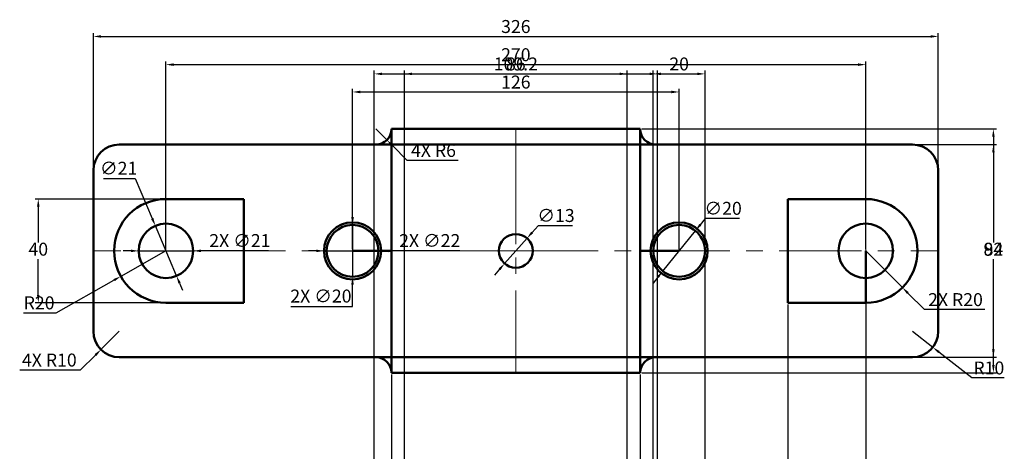
# Model space of a CAD drawing. Units: millimetres. Extents: x -44 to 350, y 28 to 429.
# Tile 2 of 2: x -44 to 336, y 262 to 429. Entities that reach past the tile are written whole.
import ezdxf

# ---------------------------------------------------------------- set-up
doc = ezdxf.new("R2010")
doc.units = ezdxf.units.MM
doc.linetypes.add('CENTER', pattern=[50.8, 31.75, -6.35, 6.35, -6.35])
for name, color, linetype, lineweight in [('M-CNTR', 1, 'CENTER', 18), ('M-DIMS', 2, 'Continuous', 25), ('M-OUTL', 7, 'Continuous', 50)]:
    doc.layers.add(name, color=color, linetype=linetype, lineweight=lineweight)
doc.styles.get("Standard").update_dxf_attribs({"font": 'arial.ttf'})
doc.dimstyles.new('ISO-25', dxfattribs={"dimtxt": 5, "dimasz": 3, "dimexe": 1.25, "dimexo": 0.625, "dimtad": 1, "dimtih": 1, "dimtoh": 1, "dimtxsty": 'Standard', "dimcen": 2.5, "dimadec": 0, "dimazin": 0, "dimtfac": 1, "dimtmove": 0, "dimatfit": 3, "dimfxl": 1, "dimarcsym": 0})

# ---------------------------------------------------------------- blocks, each defined once
blk = doc.blocks.new('*D20')
at = {"layer": 'Defpoints', "color": 0, "transparency": 16777216}
for p in [(310.7, 422.26), (-15.3, 370.57), (310.7, 370.57)]:
    blk.add_point(p, dxfattribs=at)
at = {"layer": 'M-DIMS', "color": 0, "lineweight": -2, "transparency": 16777216}
for p, q in [((-15.3, 371.19), (-15.3, 423.51)), ((-12.3, 422.26), (307.7, 422.26)), ((310.7, 371.19), (310.7, 423.51))]:
    blk.add_line(p, q, dxfattribs=at)
at = {"layer": 'M-DIMS', "color": 0, "transparency": 16777216}
for points in [[(-12.3, 422.76), (-12.3, 421.76), (-15.3, 422.26)], [(307.7, 422.76), (307.7, 421.76), (310.7, 422.26)]]:
    blk.add_solid(points, dxfattribs=at)
at = {"layer": 'M-DIMS', "color": 0, "transparency": 16777216, "insert": (147.7, 425.44), "char_height": 5, "attachment_point": 5}
blk.add_mtext('326', dxfattribs=at)
blk = doc.blocks.new('*D21')
at = {"layer": 'Defpoints', "color": 0, "transparency": 16777216}
for p in [(282.7, 411.39), (12.7, 339.57), (282.7, 339.57)]:
    blk.add_point(p, dxfattribs=at)
at = {"layer": 'M-DIMS', "color": 0, "lineweight": -2, "transparency": 16777216}
for p, q in [((12.7, 340.19), (12.7, 412.64)), ((15.7, 411.39), (279.7, 411.39)), ((282.7, 340.19), (282.7, 412.64))]:
    blk.add_line(p, q, dxfattribs=at)
at = {"layer": 'M-DIMS', "color": 0, "transparency": 16777216}
for points in [[(15.7, 411.89), (15.7, 410.89), (12.7, 411.39)], [(279.7, 411.89), (279.7, 410.89), (282.7, 411.39)]]:
    blk.add_solid(points, dxfattribs=at)
at = {"layer": 'M-DIMS', "color": 0, "transparency": 16777216, "insert": (147.7, 414.57), "char_height": 5, "attachment_point": 5}
blk.add_mtext('270', dxfattribs=at)
blk = doc.blocks.new('*D22')
at = {"layer": 'Defpoints', "color": 0, "transparency": 16777216}
for p in [(210.7, 400.84), (84.7, 339.57), (210.7, 339.57)]:
    blk.add_point(p, dxfattribs=at)
at = {"layer": 'M-DIMS', "color": 0, "lineweight": -2, "transparency": 16777216}
for p, q in [((84.7, 340.19), (84.7, 402.09)), ((87.7, 400.84), (207.7, 400.84)), ((210.7, 340.19), (210.7, 402.09))]:
    blk.add_line(p, q, dxfattribs=at)
at = {"layer": 'M-DIMS', "color": 0, "transparency": 16777216}
for points in [[(87.7, 401.34), (87.7, 400.34), (84.7, 400.84)], [(207.7, 401.34), (207.7, 400.34), (210.7, 400.84)]]:
    blk.add_solid(points, dxfattribs=at)
at = {"layer": 'M-DIMS', "color": 0, "transparency": 16777216, "insert": (147.7, 404.02), "char_height": 5, "attachment_point": 5}
blk.add_mtext('126', dxfattribs=at)
blk = doc.blocks.new('*D23')
at = {"layer": 'Defpoints', "color": 0, "transparency": 16777216}
for p in [(152.01, 344.43), (143.39, 334.7)]:
    blk.add_point(p, dxfattribs=at)
at = {"layer": 'M-DIMS', "color": 0, "lineweight": -2, "transparency": 16777216}
for p, q in [((156.27, 349.24), (154, 346.68)), ((169.5, 349.24), (156.27, 349.24)), ((143.39, 334.7), (152.01, 344.43)), ((141.4, 332.46), (139.41, 330.21))]:
    blk.add_line(p, q, dxfattribs=at)
at = {"layer": 'M-DIMS', "color": 0, "transparency": 16777216}
for points in [[(153.63, 347.01), (154.37, 346.35), (152.01, 344.43)], [(141.03, 332.79), (141.78, 332.13), (143.39, 334.7)]]:
    blk.add_solid(points, dxfattribs=at)
at = {"layer": 'M-DIMS', "color": 0, "transparency": 16777216, "insert": (163.2, 352.56), "char_height": 5, "attachment_point": 5}
blk.add_mtext('∅13', dxfattribs=at)
blk = doc.blocks.new('*D24')
at = {"layer": 'Defpoints', "color": 0, "transparency": 16777216}
for p in [(216.99, 347.34), (204.41, 331.79)]:
    blk.add_point(p, dxfattribs=at)
at = {"layer": 'M-DIMS', "color": 0, "lineweight": -2, "transparency": 16777216}
for p, q in [((220.77, 352.01), (218.88, 349.67)), ((233.98, 352.01), (220.77, 352.01)), ((204.41, 331.79), (216.99, 347.34)), ((202.52, 329.46), (200.64, 327.13))]:
    blk.add_line(p, q, dxfattribs=at)
at = {"layer": 'M-DIMS', "color": 0, "transparency": 16777216}
for points in [[(218.49, 349.99), (219.27, 349.36), (216.99, 347.34)], [(202.13, 329.78), (202.91, 329.15), (204.41, 331.79)]]:
    blk.add_solid(points, dxfattribs=at)
at = {"layer": 'M-DIMS', "color": 0, "transparency": 16777216, "insert": (227.68, 355.32), "char_height": 5, "attachment_point": 5}
blk.add_mtext('∅20', dxfattribs=at)
blk = doc.blocks.new('*D25')
at = {"layer": 'Defpoints', "color": 0, "transparency": 16777216}
for p in [(300.7, 308.57), (308.57, 302.39)]:
    blk.add_point(p, dxfattribs=at)
at = {"layer": 'M-DIMS', "color": 0, "lineweight": -2, "transparency": 16777216}
for p, q in [((300.7, 308.57), (308.57, 302.39)), ((323.61, 290.58), (310.93, 300.54)), ((336.16, 290.58), (323.61, 290.58))]:
    blk.add_line(p, q, dxfattribs=at)
at = {"layer": 'M-DIMS', "color": 0, "transparency": 16777216}
blk.add_solid([(311.23, 300.93), (310.62, 300.15), (308.57, 302.39)], dxfattribs=at)
at = {"layer": 'M-DIMS', "color": 0, "transparency": 16777216, "insert": (330.2, 293.76), "char_height": 5, "attachment_point": 5}
blk.add_mtext('R10', dxfattribs=at)
blk = doc.blocks.new('*D26')
at = {"layer": 'Defpoints', "color": 0, "transparency": 16777216}
for p in [(8.61, 349.24), (16.79, 329.9)]:
    blk.add_point(p, dxfattribs=at)
at = {"layer": 'M-DIMS', "color": 0, "lineweight": -2, "transparency": 16777216}
for p, q in [((-11.37, 367.47), (0.89, 367.47)), ((0.89, 367.47), (7.44, 352)), ((16.79, 329.9), (8.61, 349.24)), ((17.96, 327.14), (19.13, 324.37))]:
    blk.add_line(p, q, dxfattribs=at)
at = {"layer": 'M-DIMS', "color": 0, "transparency": 16777216}
for points in [[(7.9, 352.2), (6.98, 351.81), (8.61, 349.24)], [(18.42, 327.33), (17.5, 326.94), (16.79, 329.9)]]:
    blk.add_solid(points, dxfattribs=at)
at = {"layer": 'M-DIMS', "color": 0, "transparency": 16777216, "insert": (-5.55, 370.79), "char_height": 5, "attachment_point": 5}
blk.add_mtext('∅21', dxfattribs=at)
blk = doc.blocks.new('*D27')
at = {"layer": 'Defpoints', "color": 0, "transparency": 16777216}
for p in [(12.7, 339.57), (-4.72, 329.75)]:
    blk.add_point(p, dxfattribs=at)
at = {"layer": 'M-DIMS', "color": 0, "lineweight": -2, "transparency": 16777216}
for p, q in [((12.7, 339.57), (-4.72, 329.75)), ((-29.64, 315.7), (-7.34, 328.27)), ((-42.2, 315.7), (-29.64, 315.7))]:
    blk.add_line(p, q, dxfattribs=at)
at = {"layer": 'M-DIMS', "color": 0, "transparency": 16777216}
blk.add_solid([(-7.58, 328.71), (-7.09, 327.84), (-4.72, 329.75)], dxfattribs=at)
at = {"layer": 'M-DIMS', "color": 0, "transparency": 16777216, "insert": (-36.23, 318.88), "char_height": 5, "attachment_point": 5}
blk.add_mtext('R20', dxfattribs=at)
blk = doc.blocks.new('*D28')
at = {"layer": 'Defpoints', "color": 0, "transparency": 16777216}
for p in [(300.7, 380.57), (331.95, 380.57), (300.7, 298.57)]:
    blk.add_point(p, dxfattribs=at)
at = {"layer": 'M-DIMS', "color": 0, "lineweight": -2, "transparency": 16777216}
for p, q in [((301.33, 380.57), (333.2, 380.57)), ((331.95, 377.57), (331.95, 342.75)), ((331.95, 301.57), (331.95, 336.39)), ((301.33, 298.57), (333.2, 298.57))]:
    blk.add_line(p, q, dxfattribs=at)
at = {"layer": 'M-DIMS', "color": 0, "transparency": 16777216}
for points in [[(331.45, 377.57), (332.45, 377.57), (331.95, 380.57)], [(331.45, 301.57), (332.45, 301.57), (331.95, 298.57)]]:
    blk.add_solid(points, dxfattribs=at)
at = {"layer": 'M-DIMS', "color": 0, "transparency": 16777216, "insert": (331.95, 339.57), "char_height": 5, "attachment_point": 5}
blk.add_mtext('82', dxfattribs=at)
blk = doc.blocks.new('*D29')
at = {"layer": 'Defpoints', "color": 0, "transparency": 16777216}
for p in [(195.7, 386.57), (331.95, 386.57), (195.7, 292.57)]:
    blk.add_point(p, dxfattribs=at)
at = {"layer": 'M-DIMS', "color": 0, "lineweight": -2, "transparency": 16777216}
for p, q in [((196.33, 386.57), (333.2, 386.57)), ((331.95, 383.57), (331.95, 342.75)), ((331.95, 295.57), (331.95, 336.39)), ((196.33, 292.57), (333.2, 292.57))]:
    blk.add_line(p, q, dxfattribs=at)
at = {"layer": 'M-DIMS', "color": 0, "transparency": 16777216}
for points in [[(331.45, 383.57), (332.45, 383.57), (331.95, 386.57)], [(331.45, 295.57), (332.45, 295.57), (331.95, 292.57)]]:
    blk.add_solid(points, dxfattribs=at)
at = {"layer": 'M-DIMS', "color": 0, "transparency": 16777216, "insert": (331.95, 339.57), "char_height": 5, "attachment_point": 5}
blk.add_mtext('94', dxfattribs=at)
blk = doc.blocks.new('*D30')
at = {"layer": 'Defpoints', "color": 0, "transparency": 16777216}
for p in [(99.7, 292.57), (195.7, 292.57), (195.7, 28.91)]:
    blk.add_point(p, dxfattribs=at)
at = {"layer": 'M-DIMS', "color": 0, "lineweight": -2, "transparency": 16777216}
for p, q in [((99.7, 291.94), (99.7, 27.66)), ((195.7, 291.94), (195.7, 27.66)), ((102.7, 28.91), (192.7, 28.91))]:
    blk.add_line(p, q, dxfattribs=at)
at = {"layer": 'M-DIMS', "color": 0, "transparency": 16777216}
for points in [[(102.7, 29.41), (102.7, 28.41), (99.7, 28.91)], [(192.7, 29.41), (192.7, 28.41), (195.7, 28.91)]]:
    blk.add_solid(points, dxfattribs=at)
at = {"layer": 'M-DIMS', "color": 0, "transparency": 16777216, "insert": (147.7, 32.09), "char_height": 5, "attachment_point": 5}
blk.add_mtext('96', dxfattribs=at)
blk = doc.blocks.new('*D31')
at = {"layer": 'Defpoints', "color": 0, "transparency": 16777216}
for p in [(282.7, 339.57), (252.7, 319.57), (252.7, 28.91)]:
    blk.add_point(p, dxfattribs=at)
at = {"layer": 'M-DIMS', "color": 0, "lineweight": -2, "transparency": 16777216}
for p, q in [((282.7, 338.94), (282.7, 27.66)), ((252.7, 318.94), (252.7, 27.66)), ((279.7, 28.91), (255.7, 28.91))]:
    blk.add_line(p, q, dxfattribs=at)
at = {"layer": 'M-DIMS', "color": 0, "transparency": 16777216}
for points in [[(255.7, 29.41), (255.7, 28.41), (252.7, 28.91)], [(279.7, 29.41), (279.7, 28.41), (282.7, 28.91)]]:
    blk.add_solid(points, dxfattribs=at)
at = {"layer": 'M-DIMS', "color": 0, "transparency": 16777216, "insert": (267.7, 32.09), "char_height": 5, "attachment_point": 5}
blk.add_mtext('30', dxfattribs=at)
blk = doc.blocks.new('*D32')
at = {"layer": 'Defpoints', "color": 0, "transparency": 16777216}
for p in [(-36.55, 359.57), (42.7, 359.57), (42.7, 319.57)]:
    blk.add_point(p, dxfattribs=at)
at = {"layer": 'M-DIMS', "color": 0, "lineweight": -2, "transparency": 16777216}
for p, q in [((42.08, 359.57), (-37.8, 359.57)), ((-36.55, 356.57), (-36.55, 342.75)), ((-36.55, 322.57), (-36.55, 336.39)), ((42.08, 319.57), (-37.8, 319.57))]:
    blk.add_line(p, q, dxfattribs=at)
at = {"layer": 'M-DIMS', "color": 0, "transparency": 16777216}
for points in [[(-37.05, 356.57), (-36.05, 356.57), (-36.55, 359.57)], [(-37.05, 322.57), (-36.05, 322.57), (-36.55, 319.57)]]:
    blk.add_solid(points, dxfattribs=at)
at = {"layer": 'M-DIMS', "color": 0, "transparency": 16777216, "insert": (-36.55, 339.57), "char_height": 5, "attachment_point": 5}
blk.add_mtext('40', dxfattribs=at)
blk = doc.blocks.new('*D36')
at = {"layer": 'Defpoints', "color": 0, "transparency": 16777216}
for p in [(202.3, 407.82), (93.1, 177.16), (202.3, 177.16)]:
    blk.add_point(p, dxfattribs=at)
at = {"layer": 'M-DIMS', "color": 0, "lineweight": -2, "transparency": 16777216}
for p, q in [((93.1, 177.78), (93.1, 409.07)), ((96.1, 407.82), (199.3, 407.82)), ((202.3, 177.78), (202.3, 409.07))]:
    blk.add_line(p, q, dxfattribs=at)
at = {"layer": 'M-DIMS', "color": 0, "transparency": 16777216}
for points in [[(96.1, 408.32), (96.1, 407.32), (93.1, 407.82)], [(199.3, 408.32), (199.3, 407.32), (202.3, 407.82)]]:
    blk.add_solid(points, dxfattribs=at)
at = {"layer": 'M-DIMS', "color": 0, "transparency": 16777216, "insert": (147.7, 411), "char_height": 5, "attachment_point": 5}
blk.add_mtext('109.2', dxfattribs=at)
blk = doc.blocks.new('*D37')
at = {"layer": 'Defpoints', "color": 0, "transparency": 16777216}
for p in [(190.7, 407.82), (104.7, 131.22), (190.7, 131.22)]:
    blk.add_point(p, dxfattribs=at)
at = {"layer": 'M-DIMS', "color": 0, "lineweight": -2, "transparency": 16777216}
for p, q in [((104.7, 131.85), (104.7, 409.07)), ((107.7, 407.82), (187.7, 407.82)), ((190.7, 131.85), (190.7, 409.07))]:
    blk.add_line(p, q, dxfattribs=at)
at = {"layer": 'M-DIMS', "color": 0, "transparency": 16777216}
for points in [[(107.7, 408.32), (107.7, 407.32), (104.7, 407.82)], [(187.7, 408.32), (187.7, 407.32), (190.7, 407.82)]]:
    blk.add_solid(points, dxfattribs=at)
at = {"layer": 'M-DIMS', "color": 0, "transparency": 16777216, "insert": (147.7, 411), "char_height": 5, "attachment_point": 5}
blk.add_mtext('86', dxfattribs=at)
blk = doc.blocks.new('*D42')
at = {"layer": 'Defpoints', "color": 0, "transparency": 16777216}
for p in [(220.7, 407.82), (200.7, 78.16), (220.7, 78.16)]:
    blk.add_point(p, dxfattribs=at)
at = {"layer": 'M-DIMS', "color": 0, "lineweight": -2, "transparency": 16777216}
for p, q in [((200.7, 78.78), (200.7, 409.07)), ((203.7, 407.82), (217.7, 407.82)), ((220.7, 78.78), (220.7, 409.07))]:
    blk.add_line(p, q, dxfattribs=at)
at = {"layer": 'M-DIMS', "color": 0, "transparency": 16777216}
for points in [[(203.7, 408.32), (203.7, 407.32), (200.7, 407.82)], [(217.7, 408.32), (217.7, 407.32), (220.7, 407.82)]]:
    blk.add_solid(points, dxfattribs=at)
at = {"layer": 'M-DIMS', "color": 0, "transparency": 16777216, "insert": (210.7, 411), "char_height": 5, "attachment_point": 5}
blk.add_mtext('20', dxfattribs=at)
blk = doc.blocks.new('*D43')
at = {"layer": 'Defpoints', "color": 0, "transparency": 16777216}
for p in [(2.2, 339.57), (23.2, 339.57)]:
    blk.add_point(p, dxfattribs=at)
at = {"layer": 'M-DIMS', "color": 0, "lineweight": -2, "transparency": 16777216}
for p, q in [((-0.8, 339.57), (-3.8, 339.57)), ((2.2, 339.57), (23.2, 339.57)), ((29.5, 339.57), (26.2, 339.57)), ((52.33, 339.57), (29.5, 339.57))]:
    blk.add_line(p, q, dxfattribs=at)
at = {"layer": 'M-DIMS', "color": 0, "transparency": 16777216}
for points in [[(-0.8, 340.07), (-0.8, 339.07), (2.2, 339.57)], [(26.2, 340.07), (26.2, 339.07), (23.2, 339.57)]]:
    blk.add_solid(points, dxfattribs=at)
at = {"layer": 'M-DIMS', "color": 0, "transparency": 16777216, "insert": (41.23, 342.89), "char_height": 5, "attachment_point": 5}
blk.add_mtext('2X ∅21', dxfattribs=at)
blk = doc.blocks.new('*D44')
at = {"layer": 'Defpoints', "color": 0, "transparency": 16777216}
for p in [(73.7, 339.57), (95.7, 339.57)]:
    blk.add_point(p, dxfattribs=at)
at = {"layer": 'M-DIMS', "color": 0, "lineweight": -2, "transparency": 16777216}
for p, q in [((70.7, 339.57), (67.7, 339.57)), ((73.7, 339.57), (95.7, 339.57)), ((102.3, 339.57), (98.7, 339.57)), ((126.04, 339.57), (102.3, 339.57))]:
    blk.add_line(p, q, dxfattribs=at)
at = {"layer": 'M-DIMS', "color": 0, "transparency": 16777216}
for points in [[(70.7, 340.07), (70.7, 339.07), (73.7, 339.57)], [(98.7, 340.07), (98.7, 339.07), (95.7, 339.57)]]:
    blk.add_solid(points, dxfattribs=at)
at = {"layer": 'M-DIMS', "color": 0, "transparency": 16777216, "insert": (114.48, 342.89), "char_height": 5, "attachment_point": 5}
blk.add_mtext('2X ∅22', dxfattribs=at)
blk = doc.blocks.new('*D45')
at = {"layer": 'Defpoints', "color": 0, "transparency": 16777216}
for p in [(84.7, 349.57), (84.7, 329.57)]:
    blk.add_point(p, dxfattribs=at)
at = {"layer": 'M-DIMS', "color": 0, "lineweight": -2, "transparency": 16777216}
for p, q in [((84.7, 352.57), (84.7, 355.57)), ((84.7, 349.57), (84.7, 329.57)), ((84.7, 318.18), (84.7, 326.57)), ((60.93, 318.18), (84.7, 318.18))]:
    blk.add_line(p, q, dxfattribs=at)
at = {"layer": 'M-DIMS', "color": 0, "transparency": 16777216}
for points in [[(84.2, 352.57), (85.2, 352.57), (84.7, 349.57)], [(84.2, 326.57), (85.2, 326.57), (84.7, 329.57)]]:
    blk.add_solid(points, dxfattribs=at)
at = {"layer": 'M-DIMS', "color": 0, "transparency": 16777216, "insert": (72.5, 321.5), "char_height": 5, "attachment_point": 5}
blk.add_mtext('2X ∅20', dxfattribs=at)
blk = doc.blocks.new('*D46')
at = {"layer": 'Defpoints', "color": 0, "transparency": 16777216}
for p in [(282.7, 339.57), (296.84, 325.43)]:
    blk.add_point(p, dxfattribs=at)
at = {"layer": 'M-DIMS', "color": 0, "lineweight": -2, "transparency": 16777216}
for p, q in [((282.7, 339.57), (296.84, 325.43)), ((305.33, 316.94), (298.96, 323.31)), ((328.71, 316.94), (305.33, 316.94))]:
    blk.add_line(p, q, dxfattribs=at)
at = {"layer": 'M-DIMS', "color": 0, "transparency": 16777216}
blk.add_solid([(299.32, 323.66), (298.61, 322.95), (296.84, 325.43)], dxfattribs=at)
at = {"layer": 'M-DIMS', "color": 0, "transparency": 16777216, "insert": (317.33, 320.12), "char_height": 5, "attachment_point": 5}
blk.add_mtext('2X R20', dxfattribs=at)
blk = doc.blocks.new('*D47')
at = {"layer": 'Defpoints', "color": 0, "transparency": 16777216}
for p in [(-5.3, 308.57), (-12.37, 301.5)]:
    blk.add_point(p, dxfattribs=at)
at = {"layer": 'M-DIMS', "color": 0, "lineweight": -2, "transparency": 16777216}
for p, q in [((-5.3, 308.57), (-12.37, 301.5)), ((-20.22, 293.64), (-14.49, 299.38)), ((-43.72, 293.64), (-20.22, 293.64))]:
    blk.add_line(p, q, dxfattribs=at)
at = {"layer": 'M-DIMS', "color": 0, "transparency": 16777216}
blk.add_solid([(-14.85, 299.73), (-14.14, 299.02), (-12.37, 301.5)], dxfattribs=at)
at = {"layer": 'M-DIMS', "color": 0, "transparency": 16777216, "insert": (-32.29, 296.82), "char_height": 5, "attachment_point": 5}
blk.add_mtext('4X R10', dxfattribs=at)
blk = doc.blocks.new('*D48')
at = {"layer": 'Defpoints', "color": 0, "transparency": 16777216}
for p in [(93.7, 386.57), (97.94, 382.33)]:
    blk.add_point(p, dxfattribs=at)
at = {"layer": 'M-DIMS', "color": 0, "lineweight": -2, "transparency": 16777216}
for p, q in [((93.7, 386.57), (97.94, 382.33)), ((105.8, 374.47), (100.07, 380.21)), ((125.43, 374.47), (105.8, 374.47))]:
    blk.add_line(p, q, dxfattribs=at)
at = {"layer": 'M-DIMS', "color": 0, "transparency": 16777216}
blk.add_solid([(100.42, 380.56), (99.71, 379.85), (97.94, 382.33)], dxfattribs=at)
at = {"layer": 'M-DIMS', "color": 0, "transparency": 16777216, "insert": (115.92, 377.65), "char_height": 5, "attachment_point": 5}
blk.add_mtext('4X R6', dxfattribs=at)

msp = doc.modelspace()

# ---------------------------------------------------------------- linework, layer by layer
at = {"layer": 'M-CNTR'}
for p, q in [((147.7005, 292.5682), (147.7005, 386.5682)), ((147.7005, 386.5682), (147.7005, 339.5682)), ((12.7005, 380.5682), (12.7005, 339.5682)), ((84.7005, 380.5682), (84.7005, 339.5682)), ((210.7005, 380.5682), (210.7005, 339.5682)), ((282.7005, 380.5682), (282.7005, 339.5682)), ((147.7005, 339.5682), (-15.2995, 339.5682)), ((147.7005, 339.5682), (310.7005, 339.5682))]:
    msp.add_line(p, q, dxfattribs=at)
at = {"layer": 'M-OUTL'}
for p, q in [((121.0295, 386.5682), (99.7005, 386.5682)), ((99.7005, 380.5682), (99.7005, 386.5682)), ((147.7005, 386.5682), (99.7005, 386.5682)), ((147.7005, 386.5682), (121.0295, 386.5682)), ((147.7005, 386.5682), (166.4621, 386.5682)), ((147.7005, 386.5682), (195.7005, 386.5682)), ((166.4621, 386.5682), (195.7005, 386.5682)), ((195.7005, 380.5682), (195.7005, 386.5682)), ((300.7005, 380.5682), (-5.2995, 380.5682)), ((93.7005, 380.5682), (84.7005, 380.5682)), ((99.7005, 339.5682), (99.7005, 380.5682)), ((195.7005, 339.5682), (195.7005, 380.5682)), ((201.7005, 380.5682), (210.7005, 380.5682)), ((-15.2995, 370.5682), (-15.2995, 308.5682)), ((310.7005, 339.5682), (310.7005, 370.5682)), ((12.7005, 359.5682), (42.7005, 359.5682)), ((42.7005, 319.5682), (42.7005, 359.5682)), ((282.7005, 359.5682), (252.7005, 359.5682)), ((252.7005, 319.5682), (252.7005, 359.5682)), ((84.7005, 339.5682), (99.7005, 339.5682)), ((99.7005, 339.5682), (99.7005, 298.5682)), ((210.7005, 339.5682), (195.7005, 339.5682)), ((195.7005, 339.5682), (195.7005, 298.5682)), ((282.7005, 339.5682), (282.7005, 319.5682)), ((310.7005, 339.5682), (310.7005, 308.5682)), ((12.7005, 319.5682), (42.7005, 319.5682)), ((282.7005, 319.5682), (252.7005, 319.5682)), ((-5.2995, 298.5682), (93.7005, 298.5682)), ((93.7005, 298.5682), (201.7005, 298.5682)), ((99.7005, 298.5682), (99.7005, 292.5682)), ((195.7005, 298.5682), (195.7005, 292.5682)), ((300.7005, 298.5682), (201.7005, 298.5682)), ((131.6744, 292.5682), (99.7005, 292.5682)), ((99.7005, 292.5682), (99.7005, 292.5682)), ((147.7005, 292.5682), (131.6744, 292.5682)), ((147.7005, 292.5682), (163.9766, 292.5682)), ((163.9766, 292.5682), (195.7005, 292.5682)), ((195.7005, 292.5682), (195.7005, 292.5682))]:
    msp.add_line(p, q, dxfattribs=at)
for centre, radius in [((12.7005, 339.5682), 10.5), ((84.7005, 339.5682), 11), ((84.7005, 339.5682), 10), ((210.7005, 339.5682), 11), ((210.7005, 339.5682), 10), ((282.7005, 339.5682), 10.5), ((147.7005, 339.5682), 6.5)]:
    msp.add_circle(centre, radius, dxfattribs=at)
for centre, radius, start, end in [((93.7005, 386.5682), 6, 270, 0), ((201.7005, 386.5682), 6, 180, 270), ((-5.2995, 370.5682), 10, 90, 180), ((300.7005, 370.5682), 10, 0, 90), ((12.7005, 339.5682), 20, 90, 270), ((282.7005, 339.5682), 20, 270, 90), ((-5.2995, 308.5682), 10, 180, 270), ((300.7005, 308.5682), 10, 270, 0), ((93.7005, 292.5682), 6, 0, 90), ((201.7005, 292.5682), 6, 90, 180)]:
    msp.add_arc(centre, radius, start, end, dxfattribs=at)

# ---------------------------------------------------------------- dimensions: what is measured, and where the dimension line sits
at = {"layer": 'M-DIMS'}
for base, p1, p2, override, picture, middle in [((310.7005, 422.2558), (-15.2995, 370.5682), (310.7005, 370.5682), {"dimclrd": 0, "dimclre": 0, "dimclrt": 0}, '*D20', (147.7005, 425.4353)), ((282.7005, 411.392), (12.7005, 339.5682), (282.7005, 339.5682), {"dimclrd": 0, "dimclre": 0, "dimclrt": 0}, '*D21', (147.7005, 414.5699)), ((202.3037, 407.8182), (93.0974, 177.1598), (202.3037, 177.1598), {"dimdec": 1, "dimlfac": 1, "dimrnd": 0, "dimzin": 0, "dimdsep": 46, "dimlunit": 2}, '*D36', (147.7005, 410.9961)), ((190.7005, 407.8182), (104.7005, 131.2231), (190.7005, 131.2231), {"dimdec": 0, "dimlfac": 1, "dimrnd": 0, "dimzin": 0, "dimdsep": 46, "dimlunit": 2}, '*D37', (147.7005, 410.9961)), ((220.7005, 407.8182), (200.7005, 78.1598), (220.7005, 78.1598), {"dimdec": 0, "dimlfac": 1, "dimrnd": 0, "dimzin": 0, "dimdsep": 46, "dimlunit": 2}, '*D42', (210.7005, 410.9961)), ((210.7005, 400.8429), (84.7005, 339.5682), (210.7005, 339.5682), {"dimclrd": 0, "dimclre": 0, "dimclrt": 0}, '*D22', (147.7005, 404.0207)), ((252.7005, 28.9098), (282.7005, 339.5682), (252.7005, 319.5682), {"dimdec": 0, "dimlfac": 1, "dimrnd": 0, "dimzin": 0, "dimdsep": 46, "dimlunit": 2}, '*D31', (267.7005, 32.0894)), ((195.7005, 28.9098), (99.7005, 292.5682), (195.7005, 292.5682), {"dimdec": 0, "dimlfac": 1, "dimrnd": 0, "dimzin": 0, "dimdsep": 46, "dimlunit": 2}, '*D30', (147.7005, 32.0877))]:
    dim = msp.add_linear_dim(base=base, p1=p1, p2=p2, dimstyle='ISO-25', override=override, dxfattribs=at)
    dim.commit()
    dim.dimension.update_dxf_attribs({"geometry": picture, "text_midpoint": middle})
for center, mpoint, picture, middle in [((93.7005, 386.5682), (97.9438, 382.3262), '*D48', (115.925, 377.6523)), ((-5.2995, 308.5682), (-12.3707, 301.4973), '*D47', (-32.2864, 296.8224))]:
    dim = msp.add_radius_dim(center=center, mpoint=mpoint, text='4X <>', dimstyle='ISO-25', override={"dimdec": 0, "dimlfac": 1, "dimrnd": 0, "dimzin": 0, "dimdsep": 46, "dimlunit": 2}, dxfattribs=at)
    dim.commit()
    dim.dimension.update_dxf_attribs({"geometry": picture, "text_midpoint": middle})
for base, p1, p2, picture, middle in [((331.9505, 386.5682), (195.7005, 292.5682), (195.7005, 386.5682), '*D29', (331.9505, 339.5682)), ((331.9505, 380.5682), (300.7005, 298.5682), (300.7005, 380.5682), '*D28', (331.9505, 339.5682)), ((-36.5495, 359.5682), (42.7005, 319.5682), (42.7005, 359.5682), '*D32', (-36.5495, 339.5682))]:
    dim = msp.add_linear_dim(base=base, p1=p1, p2=p2, angle=90, dimstyle='ISO-25', override={"dimdec": 0, "dimlfac": 1, "dimrnd": 0, "dimzin": 0, "dimdsep": 46, "dimlunit": 2}, dxfattribs=at)
    dim.commit()
    dim.dimension.update_dxf_attribs({"geometry": picture, "text_midpoint": middle})
for p1, p2, picture, middle in [((16.7938, 329.8989), (8.6073, 349.2375), '*D26', (-5.5537, 367.4678)), ((143.3907, 334.7025), (152.0104, 344.4339), '*D23', (163.1973, 349.2442))]:
    dim = msp.add_diameter_dim_2p(p1=p1, p2=p2, dimstyle='ISO-25', override={"dimclrd": 0, "dimclre": 0, "dimclrt": 0}, dxfattribs=at)
    dim.commit()
    dim.dimension.update_dxf_attribs({"geometry": picture, "text_midpoint": middle, "dimtype": 163})
dim = msp.add_diameter_dim_2p(p1=(204.4102, 331.7944), p2=(216.9909, 347.342), dimstyle='ISO-25', override={"dimclrd": 0, "dimclre": 0, "dimclrt": 0}, dxfattribs=at)
dim.commit()
dim.dimension.update_dxf_attribs({"geometry": '*D24', "text_midpoint": (227.6827, 355.3239)})
for p1, p2, picture, middle in [((84.7011, 349.5682), (84.7, 329.5682), '*D45', (72.5004, 318.1828)), ((2.2005, 339.5664), (23.2005, 339.57), '*D43', (29.5005, 339.5711)), ((73.7005, 339.5664), (95.7005, 339.57), '*D44', (102.3005, 339.5711))]:
    dim = msp.add_diameter_dim_2p(p1=p1, p2=p2, text='2X <>', dimstyle='ISO-25', override={"dimdec": 0, "dimlfac": 1, "dimrnd": 0, "dimzin": 0, "dimdsep": 46, "dimlunit": 2}, dxfattribs=at)
    dim.commit()
    dim.dimension.update_dxf_attribs({"geometry": picture, "text_midpoint": middle, "dimtype": 163})
for center, mpoint, picture, middle in [((12.7005, 339.5682), (-4.7224, 329.7477), '*D27', (-36.2334, 315.7011)), ((300.7005, 308.5682), (308.5655, 302.3923), '*D25', (330.1998, 290.579))]:
    dim = msp.add_radius_dim(center=center, mpoint=mpoint, dimstyle='ISO-25', override={"dimclrd": 0, "dimclre": 0, "dimclrt": 0}, dxfattribs=at)
    dim.commit()
    dim.dimension.update_dxf_attribs({"geometry": picture, "text_midpoint": middle, "dimtype": 164})
dim = msp.add_radius_dim(center=(282.7005, 339.5682), mpoint=(296.8433, 325.4267), text='2X <>', dimstyle='ISO-25', override={"dimdec": 0, "dimlfac": 1, "dimrnd": 0, "dimzin": 0, "dimdsep": 46, "dimlunit": 2}, dxfattribs=at)
dim.commit()
dim.dimension.update_dxf_attribs({"geometry": '*D46', "text_midpoint": (317.3336, 316.9418), "dimtype": 164})

doc.saveas('drawing.dxf')
